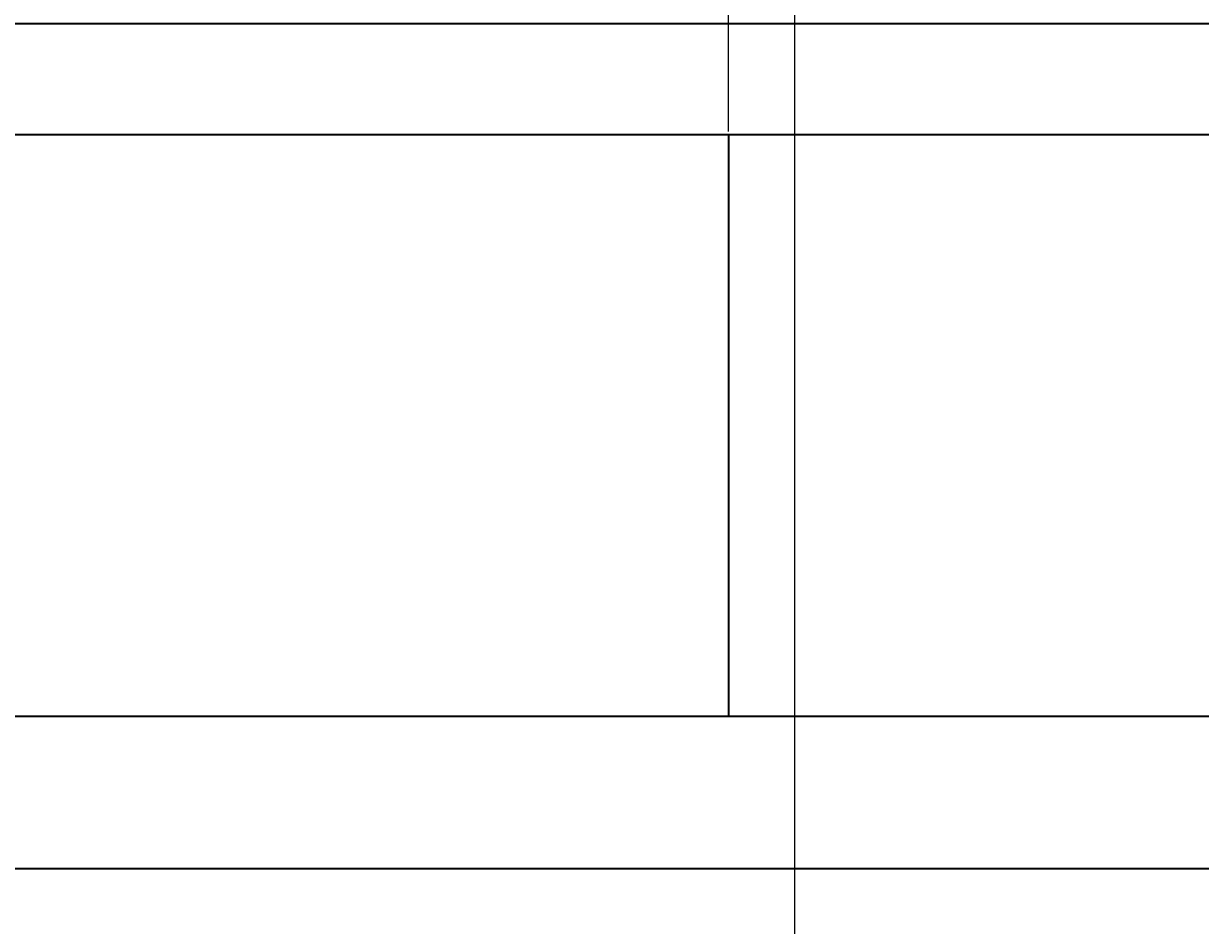
# Model space of a CAD drawing. Units: inches. Extents: x -6 to 289, y -8 to 323.
# Tile 90 of 107: x 173 to 196, y 276 to 294. Entities that reach past the tile are written whole.
import ezdxf

# ---------------------------------------------------------------- set-up
doc = ezdxf.new("R2010")
doc.units = ezdxf.units.IN
doc.header["$MEASUREMENT"] = 0
doc.layers.add('A-ANNO-DIMS', color=2, linetype='Continuous', lineweight=18)
doc.layers.add('A-ELEV', color=7, linetype='Continuous', lineweight=35)
doc.styles.get("Standard").update_dxf_attribs({"font": 'arial.ttf'})
doc.dimstyles.get("Standard").update_dxf_attribs({"dimtxt": 0.18, "dimasz": 0.18, "dimexe": 0.18, "dimexo": 0.0625, "dimgap": 0.09, "dimtad": 0, "dimtih": 1, "dimtoh": 1, "dimdec": 4, "dimzin": 0, "dimdsep": 46, "dimtxsty": 'Standard', "dimcen": 0.09, "dimadec": 0, "dimazin": 0, "dimtfac": 1, "dimtdec": 4, "dimtofl": 0, "dimtmove": 0, "dimatfit": 3, "dimfxl": 1, "dimtolj": 1, "dimtzin": 0, "dimarcsym": 0})

# ---------------------------------------------------------------- blocks, each defined once
blk = doc.blocks.new('*D12')
at = {"layer": 'A-ANNO-DIMS', "color": 0, "lineweight": -2, "transparency": 16777216}
for p, q in [((168.883, 226.717), (168.883, 322.969)), ((188.292, 226.951), (188.292, 322.969)), ((169.063, 322.789), (178.22, 322.789)), ((188.112, 322.789), (178.955, 322.789))]:
    blk.add_line(p, q, dxfattribs=at)
at = {"layer": 'A-ANNO-DIMS', "color": 0, "transparency": 16777216}
for points in [[(169.063, 322.819), (169.063, 322.759), (168.883, 322.789)], [(188.112, 322.819), (188.112, 322.759), (188.292, 322.789)]]:
    blk.add_solid(points, dxfattribs=at)
at = {"layer": 'Defpoints', "color": 0, "transparency": 16777216}
for p in [(188.292, 322.789), (188.292, 226.889), (168.883, 226.654)]:
    blk.add_point(p, dxfattribs=at)
at = {"layer": 'A-ANNO-DIMS', "color": 0, "transparency": 16777216, "insert": (178.588, 322.789), "char_height": 0.18, "attachment_point": 5}
blk.add_mtext('\\A1;19.41', dxfattribs=at)
blk = doc.blocks.new('*D13')
at = {"layer": 'A-ANNO-DIMS', "color": 0, "lineweight": -2, "transparency": 16777216}
for p, q in [((188.292, 226.951), (188.292, 322.969)), ((236.292, 226.951), (236.292, 322.969)), ((188.472, 322.789), (212.069, 322.789)), ((236.112, 322.789), (212.515, 322.789))]:
    blk.add_line(p, q, dxfattribs=at)
at = {"layer": 'A-ANNO-DIMS', "color": 0, "transparency": 16777216}
for points in [[(188.472, 322.819), (188.472, 322.759), (188.292, 322.789)], [(236.112, 322.819), (236.112, 322.759), (236.292, 322.789)]]:
    blk.add_solid(points, dxfattribs=at)
at = {"layer": 'Defpoints', "color": 0, "transparency": 16777216}
for p in [(236.292, 322.789), (188.292, 226.889), (236.292, 226.889)]:
    blk.add_point(p, dxfattribs=at)
at = {"layer": 'A-ANNO-DIMS', "color": 0, "transparency": 16777216, "insert": (212.292, 322.789), "char_height": 0.18, "attachment_point": 5}
blk.add_mtext('\\A1;48', dxfattribs=at)
blk = doc.blocks.new('*D27')
at = {"layer": 'A-ANNO-DIMS', "color": 0, "lineweight": -2, "transparency": 16777216}
for p, q in [((19.226, 307.289), (288.653, 307.289)), ((288.473, 307.109), (288.473, 277.471)), ((288.473, 247.469), (288.473, 277.107)), ((247.226, 247.289), (288.653, 247.289))]:
    blk.add_line(p, q, dxfattribs=at)
at = {"layer": 'A-ANNO-DIMS', "color": 0, "transparency": 16777216}
for points in [[(288.443, 307.109), (288.503, 307.109), (288.473, 307.289)], [(288.443, 247.469), (288.503, 247.469), (288.473, 247.289)]]:
    blk.add_solid(points, dxfattribs=at)
at = {"layer": 'Defpoints', "color": 0, "transparency": 16777216}
for p in [(19.164, 307.289), (288.473, 307.289), (247.164, 247.289)]:
    blk.add_point(p, dxfattribs=at)
at = {"layer": 'A-ANNO-DIMS', "color": 0, "transparency": 16777216, "insert": (288.473, 277.289), "char_height": 0.18, "attachment_point": 5}
blk.add_mtext('\\A1;60', dxfattribs=at)
blk = doc.blocks.new('*D79')
at = {"layer": 'A-ANNO-DIMS', "color": 0, "lineweight": -2, "transparency": 16777216}
for p, q in [((171.296, 118.033), (171.296, 322.969)), ((188.292, 116.842), (188.292, 322.969)), ((171.476, 322.789), (179.339, 322.789)), ((188.112, 322.789), (180.249, 322.789))]:
    blk.add_line(p, q, dxfattribs=at)
at = {"layer": 'A-ANNO-DIMS', "color": 0, "transparency": 16777216}
for points in [[(171.476, 322.819), (171.476, 322.759), (171.296, 322.789)], [(188.112, 322.819), (188.112, 322.759), (188.292, 322.789)]]:
    blk.add_solid(points, dxfattribs=at)
at = {"layer": 'Defpoints', "color": 0, "transparency": 16777216}
for p in [(188.292, 322.789), (171.296, 117.971), (188.292, 116.779)]:
    blk.add_point(p, dxfattribs=at)
at = {"layer": 'A-ANNO-DIMS', "color": 0, "transparency": 16777216, "insert": (179.794, 322.789), "char_height": 0.18, "attachment_point": 5}
blk.add_mtext('\\A1;16.996', dxfattribs=at)
blk = doc.blocks.new('*D80')
at = {"layer": 'A-ANNO-DIMS', "color": 0, "lineweight": -2, "transparency": 16777216}
for p, q in [((188.292, 116.842), (188.292, 322.969)), ((230.292, 116.842), (230.292, 322.969)), ((188.472, 322.789), (209.07, 322.789)), ((230.112, 322.789), (209.513, 322.789))]:
    blk.add_line(p, q, dxfattribs=at)
at = {"layer": 'A-ANNO-DIMS', "color": 0, "transparency": 16777216}
for points in [[(188.472, 322.819), (188.472, 322.759), (188.292, 322.789)], [(230.112, 322.819), (230.112, 322.759), (230.292, 322.789)]]:
    blk.add_solid(points, dxfattribs=at)
at = {"layer": 'Defpoints', "color": 0, "transparency": 16777216}
for p in [(230.292, 322.789), (188.292, 116.779), (230.292, 116.779)]:
    blk.add_point(p, dxfattribs=at)
at = {"layer": 'A-ANNO-DIMS', "color": 0, "transparency": 16777216, "insert": (209.292, 322.789), "char_height": 0.18, "attachment_point": 5}
blk.add_mtext('\\A1;42', dxfattribs=at)
blk = doc.blocks.new('*D96')
at = {"layer": 'A-ANNO-DIMS', "color": 0, "lineweight": -2, "transparency": 16777216}
for p, q in [((164.004, 159.411), (164.004, 322.969)), ((200.616, 159.411), (200.616, 322.969)), ((164.184, 322.789), (181.934, 322.789)), ((200.436, 322.789), (182.686, 322.789))]:
    blk.add_line(p, q, dxfattribs=at)
at = {"layer": 'A-ANNO-DIMS', "color": 0, "transparency": 16777216}
for points in [[(164.184, 322.819), (164.184, 322.759), (164.004, 322.789)], [(200.436, 322.819), (200.436, 322.759), (200.616, 322.789)]]:
    blk.add_solid(points, dxfattribs=at)
at = {"layer": 'Defpoints', "color": 0, "transparency": 16777216}
for p in [(200.616, 322.789), (164.004, 159.348), (200.616, 159.348)]:
    blk.add_point(p, dxfattribs=at)
at = {"layer": 'A-ANNO-DIMS', "color": 0, "transparency": 16777216, "insert": (182.31, 322.789), "char_height": 0.18, "attachment_point": 5}
blk.add_mtext('\\A1;36.61', dxfattribs=at)
blk = doc.blocks.new('*D107')
at = {"layer": 'A-ANNO-DIMS', "color": 0, "lineweight": -2, "transparency": 16777216}
for p, q in [((118.164, 293.728), (118.164, 322.969)), ((186.984, 291.541), (186.984, 322.969)), ((118.344, 322.789), (152.18, 322.789)), ((186.804, 322.789), (152.967, 322.789))]:
    blk.add_line(p, q, dxfattribs=at)
at = {"layer": 'A-ANNO-DIMS', "color": 0, "transparency": 16777216}
for points in [[(118.344, 322.819), (118.344, 322.759), (118.164, 322.789)], [(186.804, 322.819), (186.804, 322.759), (186.984, 322.789)]]:
    blk.add_solid(points, dxfattribs=at)
at = {"layer": 'Defpoints', "color": 0, "transparency": 16777216}
for p in [(186.984, 322.789), (118.164, 293.666), (186.984, 291.478)]:
    blk.add_point(p, dxfattribs=at)
at = {"layer": 'A-ANNO-DIMS', "color": 0, "transparency": 16777216, "insert": (152.574, 322.789), "char_height": 0.18, "attachment_point": 5}
blk.add_mtext('\\A1;68.82', dxfattribs=at)
blk = doc.blocks.new('*D108')
at = {"layer": 'A-ANNO-DIMS', "color": 0, "lineweight": -2, "transparency": 16777216}
for p, q in [((186.984, 291.541), (186.984, 322.969)), ((255.804, 291.541), (255.804, 322.969)), ((187.164, 322.789), (221, 322.789)), ((255.624, 322.789), (221.787, 322.789))]:
    blk.add_line(p, q, dxfattribs=at)
at = {"layer": 'A-ANNO-DIMS', "color": 0, "transparency": 16777216}
for points in [[(187.164, 322.819), (187.164, 322.759), (186.984, 322.789)], [(255.624, 322.819), (255.624, 322.759), (255.804, 322.789)]]:
    blk.add_solid(points, dxfattribs=at)
at = {"layer": 'Defpoints', "color": 0, "transparency": 16777216}
for p in [(255.804, 322.789), (186.984, 291.478), (255.804, 291.478)]:
    blk.add_point(p, dxfattribs=at)
at = {"layer": 'A-ANNO-DIMS', "color": 0, "transparency": 16777216, "insert": (221.394, 322.789), "char_height": 0.18, "attachment_point": 5}
blk.add_mtext('\\A1;68.82', dxfattribs=at)

msp = doc.modelspace()

# ---------------------------------------------------------------- linework, layer by layer
at = {"layer": 'A-ELEV'}
msp.add_line((186.9837, 291.4781), (186.9837, 280.0427), dxfattribs=at)
for points in [[(115.1638, 307.2888), (115.1638, 277.0427), (259.1638, 277.0427), (259.1638, 259.2888)], [(118.1638, 307.2888), (118.1638, 280.0427), (262.1638, 280.0427), (262.1638, 259.2888)], [(255.8036, 291.4781), (118.1638, 291.4781), (118.1638, 293.6657), (255.8036, 293.6657)]]:
    msp.add_lwpolyline(points, dxfattribs=at)

# ---------------------------------------------------------------- dimensions: what is measured, and where the dimension line sits
at = {"layer": 'A-ANNO-DIMS'}
for base, p1, p2, override, picture, middle in [((186.9837, 322.7888), (118.1638, 293.6657), (186.9837, 291.4781), {"dimdec": 2, "dimlfac": 1, "dimrnd": 0, "dimzin": 0, "dimdsep": 46, "dimlunit": 2}, '*D107', (152.5737, 322.7888)), ((200.6162, 322.7888), (164.0039, 159.3484), (200.6162, 159.3484), {"dimdec": 2, "dimlfac": 1, "dimrnd": 0, "dimzin": 0, "dimdsep": 46, "dimlunit": 2}, '*D96', (182.3101, 322.7888)), ((188.2918, 322.7888), (168.8835, 226.654), (188.2918, 226.8887), {"dimdec": 2, "dimlfac": 1, "dimrnd": 0, "dimzin": 0, "dimdsep": 46, "dimlunit": 2}, '*D12', (178.5876, 322.7888)), ((188.2918, 322.7888), (171.296, 117.9706), (188.2918, 116.7795), {"dimdec": 3, "dimlfac": 1, "dimrnd": 0, "dimzin": 0, "dimdsep": 46, "dimlunit": 2}, '*D79', (179.7939, 322.7888)), ((255.8036, 322.7888), (186.9837, 291.4781), (255.8036, 291.4781), {"dimdec": 2, "dimlfac": 1, "dimrnd": 0, "dimzin": 0, "dimdsep": 46, "dimlunit": 2}, '*D108', (221.3936, 322.7888)), ((236.2918, 322.7888), (188.2918, 226.8887), (236.2918, 226.8887), {"dimdec": 0, "dimlfac": 1, "dimrnd": 0, "dimzin": 0, "dimdsep": 46, "dimlunit": 2}, '*D13', (212.2918, 322.7888)), ((230.2918, 322.7888), (188.2918, 116.7795), (230.2918, 116.7795), {"dimdec": 0, "dimlfac": 1, "dimrnd": 0, "dimzin": 0, "dimdsep": 46, "dimlunit": 2}, '*D80', (209.2918, 322.7888))]:
    dim = msp.add_linear_dim(base=base, p1=p1, p2=p2, dimstyle='Standard', override=override, dxfattribs=at)
    dim.commit()
    dim.dimension.update_dxf_attribs({"geometry": picture, "text_midpoint": middle})
dim = msp.add_linear_dim(base=(288.4733, 307.2888), p1=(247.1638, 247.2888), p2=(19.1638, 307.2888), angle=90, dimstyle='Standard', override={"dimdec": 0, "dimlfac": 1, "dimrnd": 0, "dimzin": 0, "dimdsep": 46, "dimlunit": 2}, dxfattribs=at)
dim.commit()
dim.dimension.update_dxf_attribs({"geometry": '*D27', "text_midpoint": (288.4733, 277.2888)})

doc.saveas('drawing.dxf')
